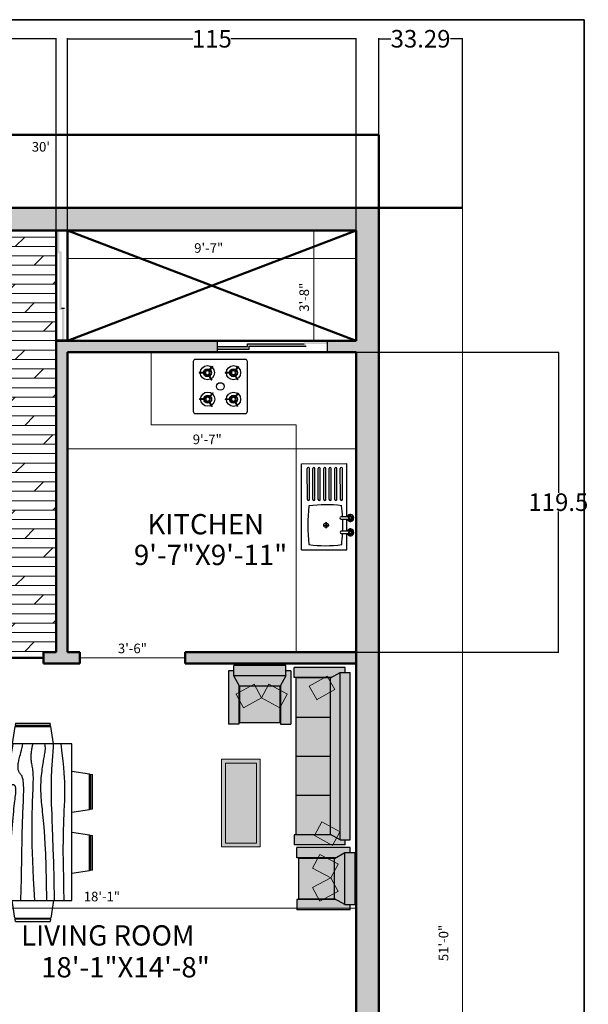
# Model space of a CAD drawing. Units: inches. Extents: x 1381 to 2246, y 1317 to 2168.
# Tile 15 of 15: x 2019 to 2246, y 1776 to 2168. Entities that reach past the tile are written whole.
import ezdxf

# ---------------------------------------------------------------- set-up
doc = ezdxf.new("R2010")
doc.units = ezdxf.units.IN
doc.header["$MEASUREMENT"] = 0
doc.layers.get('0').update_dxf_attribs({"color": 253})
for name, color, linetype, lineweight in [('A-ANNO-DIMS', 2, 'Continuous', 18), ('A-ANNO-TEXT', 7, 'Continuous', 18), ('A-ANNO-TTLB', 7, 'Continuous', 35), ('A-AREA-IDEN', 3, 'Continuous', 25), ('A-FLOR-FIXT', 9, 'Continuous', 18), ('A-FLOR-PATT', 252, 'Continuous', 13), ('A-FURN', 8, 'Continuous', 18), ('A-GLAZ', 4, 'Continuous', 25), ('A-WALL', 7, 'Continuous', 50), ('A-WALL-PATT', 8, 'Continuous', 13)]:
    doc.layers.add(name, color=color, linetype=linetype, lineweight=lineweight)
doc.layers.add('furniture', color=250, linetype='Continuous')
doc.styles.get("Standard").update_dxf_attribs({"font": 'arial.ttf'})
doc.dimstyles.get("Standard").update_dxf_attribs({"dimtxt": 7, "dimasz": 0.18, "dimexe": 0.18, "dimexo": 0.0625, "dimgap": 0.09, "dimtad": 0, "dimtih": 1, "dimtoh": 1, "dimdec": 1, "dimzin": 0, "dimdsep": 46, "dimlunit": 3, "dimtxsty": 'Standard', "dimcen": 0.09, "dimadec": 0, "dimazin": 0, "dimtfac": 1, "dimtdec": 1, "dimtofl": 0, "dimtmove": 0, "dimatfit": 3, "dimfxl": 1, "dimtolj": 1, "dimtzin": 0, "dimarcsym": 0})

# ---------------------------------------------------------------- blocks, each defined once
blk = doc.blocks.new('4bstove')
at = {"layer": 'furniture'}
for p, q in [((1452.73, 1446.21), (1452.73, 1448.61)), ((1452.98, 1446.22), (1452.98, 1448.61)), ((1464.44, 1446.34), (1464.44, 1448.73)), ((1464.69, 1446.34), (1464.69, 1448.73)), ((1451.74, 1444.45), (1449.67, 1443.25)), ((1451.87, 1444.23), (1449.79, 1443.04)), ((1453.75, 1444.08), (1455.58, 1442.54)), ((1453.91, 1444.27), (1455.74, 1442.73)), ((1463.45, 1444.58), (1461.38, 1443.38)), ((1463.57, 1444.36), (1461.5, 1443.17)), ((1465.46, 1444.21), (1467.29, 1442.67)), ((1465.62, 1444.4), (1467.45, 1442.86)), ((1452.69, 1434.81), (1452.69, 1437.2)), ((1452.94, 1434.81), (1452.94, 1437.2)), ((1464.44, 1434.81), (1464.44, 1437.2)), ((1464.69, 1434.81), (1464.69, 1437.2)), ((1451.7, 1433.04), (1449.63, 1431.85)), ((1451.82, 1432.83), (1449.75, 1431.63)), ((1453.71, 1432.67), (1455.54, 1431.13)), ((1453.87, 1432.86), (1455.7, 1431.33)), ((1463.45, 1433.04), (1461.38, 1431.85)), ((1463.57, 1432.83), (1461.5, 1431.63)), ((1465.46, 1432.67), (1467.29, 1431.13)), ((1465.62, 1432.86), (1467.45, 1431.33))]:
    blk.add_line(p, q, dxfattribs=at)
for points in [[(1447.5, 1427.38), (1469.5, 1427.38, 0.414214), (1470.5, 1428.38), (1470.5, 1450.38, 0.414214), (1469.5, 1451.38), (1447.5, 1451.38, 0.414214), (1446.5, 1450.38), (1446.5, 1428.38, 0.414214)], [(1453.75, 1444.97, 1), (1452, 1444.97, 1)], [(1465.46, 1445.1, 1), (1463.71, 1445.1, 1)], [(1453.71, 1433.56, 1), (1451.96, 1433.56, 1)], [(1465.46, 1433.56, 1), (1463.71, 1433.56, 1)]]:
    blk.add_lwpolyline(points, format="xyb", close=True, dxfattribs=at)
for points in [[(1454.12, 1444.97, 1), (1451.62, 1444.97, 1), (1454.12, 1444.97, 1)], [(1465.83, 1445.1, 1), (1463.33, 1445.1, 1), (1465.83, 1445.1, 1)], [(1454.08, 1433.56, 1), (1451.58, 1433.56, 1), (1454.08, 1433.56, 1)], [(1465.83, 1433.56, 1), (1463.33, 1433.56, 1), (1465.83, 1433.56, 1)]]:
    blk.add_lwpolyline(points, format="xyb", dxfattribs=at)
for centre, radius in [((1452.87, 1444.97), 3.14), ((1452.87, 1444.97), 1.75), ((1464.58, 1445.1), 3.14), ((1464.58, 1445.1), 1.75), ((1458.5, 1439.38), 1.67), ((1452.83, 1433.56), 3.14), ((1452.83, 1433.56), 1.75), ((1464.58, 1433.56), 3.14), ((1464.58, 1433.56), 1.75)]:
    blk.add_circle(centre, radius, dxfattribs=at)
for centre, start, end in [((1452.87, 1444.97), 88.2645, 92.2039), ((1464.58, 1445.1), 88.2645, 92.2039), ((1452.87, 1444.97), 208.188, 212.1274), ((1452.87, 1444.97), 318.1018, 322.0412), ((1464.58, 1445.1), 208.188, 212.1274), ((1464.58, 1445.1), 318.1018, 322.0412), ((1452.83, 1433.56), 88.2645, 92.2039), ((1464.58, 1433.56), 88.2645, 92.2039)]:
    blk.add_arc(centre, 3.64, start, end, dxfattribs=at)
blk = doc.blocks.new('stove')
at = {"layer": 'furniture', "xscale": 0.9, "yscale": 0.9, "zscale": 0.9, "rotation": 89.99999999999999}
blk.add_blockref('4bstove', (1295.44, -1312.65), dxfattribs=at)
blk = doc.blocks.new('A$C799204C7')
for p, q in [((0, 34.2), (17.99, 34.2)), ((0, 0), (0, 34.2)), ((2.32, 20.01), (2.32, 32.27)), ((3.13, 20.01), (3.13, 32.27)), ((4.48, 20.01), (4.48, 32.27)), ((5.29, 20.01), (5.29, 32.27)), ((6.64, 20.01), (6.64, 32.27)), ((7.45, 20.01), (7.45, 32.27)), ((8.85, 20.01), (8.85, 32.27)), ((9.66, 20.01), (9.66, 32.27)), ((11.01, 20.01), (11.01, 32.27)), ((11.82, 20.01), (11.82, 32.27)), ((13.22, 20.01), (13.22, 32.27)), ((14.03, 20.01), (14.03, 32.27)), ((15.42, 20.01), (15.42, 32.27)), ((16.24, 20.01), (16.24, 32.27)), ((17.99, 13.08), (17.99, 34.2)), ((18.59, 13.08), (15.71, 13.08)), ((15.71, 12.17), (18.59, 12.17)), ((17.99, 7.36), (17.99, 12.17)), ((8.52, 9.77), (10.9, 9.77)), ((9.73, 11), (9.73, 8.54)), ((18.59, 7.36), (15.71, 7.36)), ((15.71, 6.45), (18.59, 6.45)), ((17.99, 0), (17.99, 6.45)), ((0, 0), (17.99, 0))]:
    blk.add_line(p, q)
for centre, radius in [((19.38, 12.62), 0.684), ((19.38, 12.62), 0.456), ((9.7, 9.77), 0.916), ((19.38, 6.91), 0.684), ((19.38, 6.91), 0.456)]:
    blk.add_circle(centre, radius)
for centre, radius, start, end in [((2.72, 32.27), 0.407, 0, 180), ((4.88, 32.27), 0.407, 0, 180), ((7.05, 32.27), 0.407, 0, 180), ((9.25, 32.27), 0.407, 0, 180), ((11.42, 32.27), 0.407, 0, 180), ((13.62, 32.27), 0.407, 0, 180), ((15.83, 32.27), 0.407, 0, 180), ((2.72, 20.01), 0.407, 180, 0), ((4.88, 20.01), 0.407, 180, 0), ((7.05, 20.01), 0.407, 180, 0), ((9.25, 20.01), 0.407, 180, 0), ((11.42, 20.01), 0.407, 180, 0), ((13.62, 20.01), 0.407, 180, 0), ((15.83, 20.01), 0.407, 180, 0), ((67.33, 9.77), 64.88, 173.1952, 186.8048), ((9.53, -30.19), 48.1, 82.3437, 97.8966), ((-48.51, 9.77), 64.88, 2.9208, 6.8048), ((15.71, 12.62), 0.456, 90, 270), ((-48.51, 9.77), 64.88, 357.8723, 2.115), ((19.38, 12.62), 1.37, 199.6514, 160.3603), ((19.38, 12.62), 0.911, 210.3431, 149.7554), ((19.38, 6.91), 1.37, 199.6514, 160.3603), ((19.38, 6.91), 0.911, 210.3431, 149.7554), ((15.71, 6.91), 0.456, 90, 270), ((-48.51, 9.77), 64.88, 353.1952, 357.0665), ((9.53, 49.73), 48.1, 262.1034, 277.6563)]:
    blk.add_arc(centre, radius, start, end)
blk = doc.blocks.new('sink')
at = {"layer": 'furniture'}
for p, q in [((8718164202.684322, -1433730581.131674), (8718164202.684322, -1433730583.598095)), ((8718164203.894819, -1433730582.369047), (8718164201.504578, -1433730582.369047)), ((8718164196.150837, -1433730592.638258), (8718164196.150837, -1433730604.938997)), ((8718164196.967728, -1433730592.638258), (8718164196.967728, -1433730604.938997)), ((8718164198.365185, -1433730592.638258), (8718164198.365185, -1433730604.938997)), ((8718164199.182076, -1433730592.638258), (8718164199.182076, -1433730604.938997)), ((8718164200.579533, -1433730592.638258), (8718164200.579533, -1433730604.938997)), ((8718164201.396423, -1433730592.638258), (8718164201.396423, -1433730604.938997)), ((8718164202.748692, -1433730592.638258), (8718164202.748692, -1433730604.938997)), ((8718164203.565582, -1433730592.638258), (8718164203.565582, -1433730604.938997)), ((8718164204.963041, -1433730592.638258), (8718164204.963041, -1433730604.938997)), ((8718164205.779934, -1433730592.638258), (8718164205.779934, -1433730604.938997)), ((8718164207.1322, -1433730592.638258), (8718164207.1322, -1433730604.938997)), ((8718164207.949093, -1433730592.638258), (8718164207.949093, -1433730604.938997)), ((8718164209.301359, -1433730592.638258), (8718164209.301359, -1433730604.938997)), ((8718164210.118252, -1433730592.638258), (8718164210.118252, -1433730604.938997))]:
    blk.add_line(p, q, dxfattribs=at)
for centre, radius in [((8718164192.998869, -1433730579.495552), 0.685789), ((8718164192.998869, -1433730579.495552), 0.457192), ((8718164202.715019, -1433730582.369047), 0.919003), ((8718164192.998869, -1433730585.228166), 0.68579), ((8718164192.998869, -1433730585.228166), 0.68579), ((8718164192.998869, -1433730585.228166), 0.457192)]:
    blk.add_circle(centre, radius, dxfattribs=at)
for centre, radius, start, end in [((8718164196.559284, -1433730592.638258), 0.41045, 354.3355999, 185.6644001), ((8718164198.77363, -1433730592.638258), 0.41045, 354.3355999, 185.6644001), ((8718164200.98798, -1433730592.638258), 0.41045, 354.3355999, 185.6644001), ((8718164203.157139, -1433730592.638258), 0.41045, 354.3355999, 185.6644001), ((8718164205.371487, -1433730592.638258), 0.41045, 354.3355999, 185.6644001), ((8718164207.540646, -1433730592.640262), 0.41045, 354.3355999, 185.6644001), ((8718164209.709805, -1433730592.640262), 0.41045, 354.3355999, 185.6644001), ((8718164196.559284, -1433730604.938997), 0.408445, 180, 0), ((8718164198.77363, -1433730604.938997), 0.408445, 180, 0), ((8718164200.98798, -1433730604.938997), 0.408445, 180, 0), ((8718164203.157139, -1433730604.938997), 0.408445, 180, 0), ((8718164205.371487, -1433730604.938997), 0.408445, 180, 0), ((8718164207.540646, -1433730604.938997), 0.408445, 180, 0), ((8718164209.709805, -1433730604.938997), 0.408445, 180, 0)]:
    blk.add_arc(centre, radius, start, end, dxfattribs=at)
at = {"layer": 'furniture', "xscale": 1.0032, "yscale": 1.0032, "zscale": 1.0032, "rotation": 180}
blk.add_blockref('A$C799204C7', (8718164212.441259, -1433730572.566334), dxfattribs=at)
blk = doc.blocks.new('washbasin')
at = {"layer": 'furniture'}
blk.add_blockref('sink', (-8718164214.119328, 1433730589.721069), dxfattribs=at)
blk = doc.blocks.new('Dining Set - 36 x 72 in.')
for p, q in [((-22, 27.5), (-22.1562, 26.50042)), ((-22, 27.5), (-6, 27.5)), ((-5.8437, 26.49966), (-6, 27.5)), ((6, 27.5), (5.8438, 26.50042)), ((6, 27.5), (22, 27.5)), ((22.1563, 26.49966), (22, 27.5)), ((-22.2343, 26.00059), (-23.4847, 17.99762)), ((-22.2304, 26), (-5.7608, 26)), ((-5.8416, 26.5), (-22.1534, 26.5)), ((-4.5152, 17.99762), (-5.7655, 25.99926)), ((5.7657, 26.00059), (4.5153, 17.99762)), ((5.7696, 26), (22.2392, 26)), ((22.1584, 26.5), (5.8466, 26.5)), ((23.4848, 17.99762), (22.2345, 25.99926)), ((36, 18), (-36, 18)), ((-36, 18), (-36, -18)), ((36, -18), (36, 18)), ((-44.0006, 8.23428), (-35.9976, 9.48474)), ((44.0006, 8.23428), (35.9976, 9.48474)), ((-45.5, 8), (-44.5004, 8.15617)), ((-45.5, 8), (-45.5, -8)), ((-44.5, -8.15843), (-44.5, 8.15338)), ((-44, 8.23041), (-44, -8.23915)), ((44, 8.23041), (44, -8.23915)), ((44.5, -8.15843), (44.5, 8.15338)), ((45.5, 8), (44.5005, 8.15617)), ((45.5, 8), (45.5, -8)), ((-44.4997, -8.15631), (-45.5, -8)), ((-35.9976, -9.48476), (-43.9993, -8.2345)), ((35.9976, -9.48476), (43.9993, -8.2345)), ((44.4997, -8.15631), (45.5, -8)), ((-36, -18), (36, -18)), ((-22.2343, -26.0006), (-23.4847, -17.99762)), ((-4.5152, -17.99762), (-5.7655, -25.99928)), ((5.7657, -26.0006), (4.5153, -17.99762)), ((23.4848, -17.99762), (22.2345, -25.99928)), ((-22.2304, -26), (-5.7608, -26)), ((-22, -27.5), (-22.1562, -26.50044)), ((-5.8416, -26.5), (-22.1534, -26.5)), ((-5.8437, -26.49967), (-6, -27.5)), ((5.7696, -26), (22.2392, -26)), ((6, -27.5), (5.8438, -26.50044)), ((22.1584, -26.5), (5.8466, -26.5)), ((22.1563, -26.49967), (22, -27.5)), ((-22, -27.5), (-6, -27.5)), ((6, -27.5), (22, -27.5))]:
    blk.add_line(p, q)
for points in [[(-36, 15), (-31.1772, 14.97754), (-26.8079, 14.91406), (-22.8538, 14.81543), (-19.276, 14.6875), (-16.0362, 14.53613), (-13.0957, 14.36718), (-10.4159, 14.18652), (-7.9583, 14), (-5.6904, 13.81315), (-3.6035, 13.63021), (-1.6954, 13.45508), (0.0365, 13.29166), (1.5945, 13.14388), (2.9811, 13.01562), (4.1988, 12.9108), (5.25, 12.83333), (6.1393, 12.78613), (6.8802, 12.76823), (7.4883, 12.77767), (7.9792, 12.8125), (8.3685, 12.87077), (8.6719, 12.95052), (8.9049, 13.0498), (9.0833, 13.16666), (9.2205, 13.29899), (9.3216, 13.44401), (9.3895, 13.59879), (9.4271, 13.76041), (9.4373, 13.92594), (9.4232, 14.09245), (9.3875, 14.257), (9.3333, 14.41666), (9.2638, 14.56917), (9.1836, 14.71484), (9.0975, 14.85465), (9.0104, 14.98958), (8.9272, 15.1206), (8.8529, 15.2487), (8.7922, 15.37483), (8.75, 15.5), (8.7305, 15.62467), (8.7344, 15.74739), (8.7617, 15.86621), (8.8125, 15.97916), (8.8867, 16.08431), (8.9844, 16.17968), (9.1055, 16.26334), (9.25, 16.33333), (9.4189, 16.38802), (9.6172, 16.42708), (9.8506, 16.45052), (10.125, 16.45833), (10.4463, 16.45052), (10.8203, 16.42708), (11.2529, 16.38802), (11.75, 16.33333), (12.3184, 16.26318), (12.9694, 16.17838), (13.7151, 16.07991), (14.5677, 15.96875), (15.5395, 15.84586), (16.6426, 15.71224), (17.8893, 15.56884), (19.2917, 15.41666), (20.859, 15.25667), (22.5879, 15.08984), (24.4721, 14.91715), (26.5052, 14.73958), (28.6809, 14.5581), (30.9929, 14.3737), (33.4347, 14.18733), (36, 14)], [(-36, 10), (-28.9766, 10.14274), (-23.1725, 10.20442), (-18.4241, 10.19775), (-14.5677, 10.13541), (-11.4399, 10.03011), (-8.877, 9.89453), (-6.7154, 9.74137), (-4.7917, 9.58333), (-2.9698, 9.43082), (-1.2246, 9.28515), (0.4415, 9.14534), (2.026, 9.01041), (3.5266, 8.87939), (4.9408, 8.7513), (6.266, 8.62516), (7.5, 8.5), (8.6411, 8.37549), (9.6914, 8.2539), (10.6538, 8.13818), (11.5312, 8.03125), (12.3267, 7.93603), (13.043, 7.85547), (13.6831, 7.79248), (14.25, 7.75), (14.7471, 7.7303), (15.1797, 7.73307), (15.5537, 7.75732), (15.875, 7.80208), (16.1494, 7.86637), (16.3828, 7.94922), (16.5811, 8.04964), (16.75, 8.16666), (16.8944, 8.29915), (17.0143, 8.44531), (17.1089, 8.60319), (17.1771, 8.77083), (17.218, 8.94629), (17.2305, 9.1276), (17.2137, 9.31282), (17.1667, 9.5), (17.0895, 9.6875), (16.987, 9.875), (16.8649, 10.0625), (16.7292, 10.25), (16.5856, 10.4375), (16.4401, 10.625), (16.2985, 10.8125), (16.1667, 11), (16.05, 11.18733), (15.9518, 11.3737), (15.8752, 11.5581), (15.8229, 11.73958), (15.798, 11.91715), (15.8034, 12.08984), (15.842, 12.25667), (15.9167, 12.41666), (16.0295, 12.56836), (16.1784, 12.70833), (16.3605, 12.83268), (16.5729, 12.9375), (16.8127, 13.01888), (17.0768, 13.07291), (17.3625, 13.0957), (17.6667, 13.08333), (17.9894, 13.03312), (18.3418, 12.94726), (18.7382, 12.82918), (19.1927, 12.68229), (19.7195, 12.51001), (20.3327, 12.31575), (21.0465, 12.10294), (21.875, 11.875), (22.8357, 11.63354), (23.959, 11.37304), (25.2786, 11.08618), (26.8282, 10.76562), (28.6414, 10.40405), (30.752, 9.99414), (33.1936, 9.52856), (36, 9)], [(-36, 5.5), (-30.7157, 5.3348), (-26.069, 5.20963), (-21.9946, 5.11767), (-18.4271, 5.05208), (-15.3009, 5.00602), (-12.5508, 4.97265), (-10.1112, 4.94515), (-7.9167, 4.91666), (-5.909, 4.88167), (-4.0586, 4.83984), (-2.3429, 4.79215), (-0.7396, 4.73958), (0.7739, 4.6831), (2.22, 4.6237), (3.6213, 4.56233), (5, 4.5), (6.373, 4.43782), (7.7344, 4.3776), (9.0723, 4.32129), (10.375, 4.27083), (11.6309, 4.22819), (12.8281, 4.19531), (13.9551, 4.17415), (15, 4.16666), (15.954, 4.17448), (16.819, 4.19791), (17.6001, 4.23698), (18.3021, 4.29166), (18.9299, 4.36198), (19.4883, 4.44791), (19.9823, 4.54948), (20.4167, 4.66666), (20.7969, 4.79899), (21.1302, 4.94401), (21.4245, 5.09879), (21.6875, 5.26041), (21.9271, 5.42594), (22.1511, 5.59245), (22.3672, 5.757), (22.5834, 5.91666), (22.8065, 6.06868), (23.0404, 6.21093), (23.2879, 6.34147), (23.5521, 6.45833), (23.8358, 6.55957), (24.142, 6.64323), (24.4735, 6.70735), (24.8334, 6.75), (25.2235, 6.76969), (25.642, 6.76692), (26.0858, 6.74267), (26.5521, 6.69791), (27.0379, 6.63362), (27.5404, 6.55078), (28.0565, 6.45036), (28.5834, 6.33333), (29.1242, 6.19987), (29.7071, 6.04687), (30.3661, 5.87044), (31.1354, 5.66666), (32.0493, 5.43164), (33.142, 5.16146), (34.4475, 4.85221), (36, 4.5)], [(-36, -1), (-30.7915, -0.6591), (-26.0195, -0.38216), (-21.6519, -0.16284), (-17.6563, 0.00521), (-14.0005, 0.12833), (-10.6523, 0.21289), (-7.5796, 0.26522), (-4.75, 0.29166), (-2.134, 0.29793), (0.2878, 0.28711), (2.5317, 0.26163), (4.6146, 0.22396), (6.5529, 0.17651), (8.3633, 0.12174), (10.0623, 0.06209), (11.6667, 0), (13.1899, -0.06201), (14.6341, -0.1211), (15.9982, -0.17432), (17.2813, -0.21875), (18.4823, -0.25147), (19.6003, -0.26953), (20.6343, -0.27002), (21.5834, -0.25), (22.4481, -0.20768), (23.2357, -0.14584), (23.9549, -0.06836), (24.6146, 0.02083), (25.2235, 0.11784), (25.7904, 0.21875), (26.3241, 0.31966), (26.8334, 0.41666), (27.3265, 0.50618), (27.8099, 0.58593), (28.2894, 0.65397), (28.7709, 0.70833), (29.2601, 0.74707), (29.763, 0.76823), (30.2855, 0.76985), (30.8334, 0.75), (31.4088, 0.70784), (31.9994, 0.64713), (32.589, 0.57275), (33.1615, 0.48958), (33.7008, 0.4025), (34.1908, 0.3164), (34.6153, 0.23616), (34.9584, 0.16666), (35.2099, 0.11165), (35.3848, 0.07031), (35.504, 0.04069), (35.5886, 0.02083), (35.6594, 0.00879), (35.7377, 0.0026), (35.8442, 0.00032), (36, 0)], [(-36, -6.5), (-27.1843, -6.31267), (-20.084, -6.1263), (-14.469, -5.9419), (-10.1094, -5.76042), (-6.7752, -5.58285), (-4.2363, -5.41016), (-2.2629, -5.24333), (-0.625, -5.08334), (0.8708, -4.93099), (2.2715, -4.78646), (3.5872, -4.64974), (4.8281, -4.52084), (6.0046, -4.39974), (7.127, -4.28646), (8.2053, -4.18099), (9.25, -4.08334), (10.2705, -3.99382), (11.2734, -3.91407), (12.2647, -3.84603), (13.25, -3.79167), (14.2354, -3.75293), (15.2266, -3.73177), (16.2295, -3.73015), (17.25, -3.75), (18.2912, -3.79248), (19.3451, -3.85547), (20.4009, -3.93604), (21.4479, -4.03125), (22.4754, -4.13819), (23.4727, -4.25391), (24.4289, -4.37549), (25.3334, -4.5), (26.1785, -4.62492), (26.9694, -4.74935), (27.7145, -4.87281), (28.4219, -4.99479), (29.1, -5.11483), (29.7572, -5.23242), (30.4016, -5.34709), (31.0417, -5.45834), (31.6837, -5.56437), (32.3262, -5.65821), (32.9658, -5.73153), (33.599, -5.77604), (34.2224, -5.78345), (34.8327, -5.74545), (35.4264, -5.65373), (36, -5.5)], [(-36, -10), (-26.4022, -9.81299), (-18.4675, -9.62891), (-11.9839, -9.45069), (-6.7396, -9.28125), (-2.5226, -9.12354), (0.8789, -8.98047), (3.6769, -8.85498), (6.0833, -8.75), (8.2767, -8.66765), (10.3021, -8.60677), (12.1712, -8.56543), (13.8958, -8.54167), (15.4876, -8.53353), (16.9583, -8.53907), (18.3197, -8.55632), (19.5834, -8.58334), (20.7616, -8.61841), (21.8685, -8.66081), (22.9188, -8.71004), (23.9271, -8.76563), (24.9081, -8.82707), (25.8763, -8.89388), (26.8465, -8.96558), (27.8334, -9.04167), (28.8474, -9.12118), (29.8828, -9.20117), (30.93, -9.27824), (31.9792, -9.34896), (33.0205, -9.40991), (34.0443, -9.45768), (35.0407, -9.48885), (36, -9.5)], [(-36, -14.5), (-30.0881, -14.33513), (-25.0332, -14.21224), (-20.7312, -14.12647), (-17.0781, -14.07292), (-13.97, -14.04671), (-11.3027, -14.04297), (-8.9724, -14.05681), (-6.875, -14.08334), (-4.9224, -14.11833), (-3.0905, -14.16016), (-1.3709, -14.20785), (0.2448, -14.26042), (1.7647, -14.3169), (3.1973, -14.3763), (4.5507, -14.43767), (5.8333, -14.5), (7.0554, -14.5621), (8.235, -14.62175), (9.3922, -14.67652), (10.5469, -14.72396), (11.7192, -14.76164), (12.929, -14.78711), (14.1965, -14.79794), (15.5417, -14.79167), (16.9933, -14.76424), (18.6152, -14.70508), (20.4804, -14.60197), (22.6615, -14.44271), (25.2312, -14.21509), (28.2624, -13.9069), (31.8277, -13.50594), (36, -13)]]:
    blk.add_lwpolyline(points)
blk = doc.blocks.new('dining area')
at = {"layer": 'furniture', "xscale": 0.6659924291999282, "yscale": 0.6659924291999282, "zscale": 0.6659924291999282, "rotation": 90}
blk.add_blockref('Dining Set - 36 x 72 in.', (-0.44, 20.51), dxfattribs=at)
blk = doc.blocks.new('FABRIC SOFA 4S')
at = {"layer": 'furniture'}
for p, q in [((3, 54), (34, 54)), ((3, 51), (3, 54)), ((34, 48), (34, 54)), ((0, -51), (0, 51)), ((6, 51), (0, 51)), ((6, -51), (6, 51)), ((12, 47.63), (6, 51)), ((11.14, 48), (34, 48)), ((33, 23.81), (12, 23.81)), ((33, 0), (12, 0)), ((33, -23.81), (12, -23.81)), ((6, -51), (12, -47.63)), ((6, -51), (0, -51)), ((3, -54), (3, -51)), ((11.54, -48), (34, -48)), ((34, -48), (34, -54)), ((3, -54), (34, -54))]:
    blk.add_line(p, q, dxfattribs=at)
blk.add_lwpolyline([(12, -47.63), (12, 47.63), (33, 47.63), (33, -47.63)], close=True, dxfattribs=at)
blk = doc.blocks.new('FABRIC SOFA 1S')
at = {"layer": 'furniture'}
for p, q in [((3, 18.12), (34, 18.12)), ((3, 15.12), (3, 18.12)), ((34, 12.12), (34, 18.12)), ((0, -15.12), (0, 15.12)), ((6, 15.12), (0, 15.12)), ((6, -15.12), (6, 15.12)), ((12, 11.75), (6, 15.12)), ((11.33, 12.12), (34, 12.12)), ((6, -15.12), (0, -15.12)), ((3, -18.12), (3, -15.12)), ((6, -15.12), (12, -11.75)), ((11.33, -12.12), (34, -12.12)), ((34, -12.12), (34, -18.12)), ((3, -18.12), (34, -18.12))]:
    blk.add_line(p, q, dxfattribs=at)
blk.add_lwpolyline([(12, -11.75), (12, 11.75), (33, 11.75), (33, -11.75)], close=True, dxfattribs=at)
blk = doc.blocks.new('TV-UNIT')
for p, q in [((0, 5.36), (7.38, 9.32)), ((7.38, 9.32), (10.3, 3.88)), ((13.22, 9.32), (10.3, 3.88)), ((20.6, 5.36), (13.22, 9.32)), ((3.07, 0), (0.15, 5.44)), ((17.53, 0), (20.45, 5.44)), ((10.3, 3.88), (3.07, 0)), ((10.3, 3.88), (17.53, 0))]:
    blk.add_line(p, q)
blk = doc.blocks.new('WALL-UNIT')
for p, q in [((2.92, 18.64), (0, 13.2)), ((10.3, 14.68), (2.92, 18.64)), ((0, 13.2), (7.23, 9.32)), ((7.23, 9.32), (10.15, 14.76)), ((0, 5.44), (7.23, 9.32)), ((7.23, 9.32), (10.15, 3.88)), ((2.92, 0), (0, 5.44)), ((10.3, 3.96), (2.92, 0))]:
    blk.add_line(p, q)
blk = doc.blocks.new('SOFA-CUSHION')
for p, q in [((2.92, 9.32), (0, 3.88)), ((10.3, 5.36), (2.92, 9.32)), ((7.23, 0), (10.15, 5.44)), ((0, 3.88), (7.23, 0))]:
    blk.add_line(p, q)
blk = doc.blocks.new('WIN-KITCHEN')
for p, q in [((0, 0), (0, 4.5)), ((0, 4.5), (43.68, 4.5)), ((43.68, 4.5), (43.68, 0)), ((43.68, 0), (0, 0))]:
    blk.add_line(p, q)
blk = doc.blocks.new('CENTER-TABLE')
for p, q in [((0, 0), (0, 34.91)), ((0, 34.91), (15.37, 34.91)), ((15.37, 34.91), (15.37, 0)), ((15.37, 0), (0, 0))]:
    blk.add_line(p, q)
blk = doc.blocks.new('SIDE-TABLE')
for p, q in [((0, 0), (0, 31.87)), ((0, 31.87), (12.34, 31.87)), ((12.34, 31.87), (12.34, 0)), ((12.34, 0), (0, 0))]:
    blk.add_line(p, q)
blk = doc.blocks.new('*D78')
at = {"layer": 'A-ANNO-DIMS', "color": 0, "lineweight": -2, "transparency": 16777216}
for p, q in [((2162.31, 2092.98), (2162.31, 2160.41)), ((2162.49, 2160.23), (2167.04, 2160.23)), ((2195.41, 2160.23), (2190.86, 2160.23)), ((2195.59, 2092.98), (2195.59, 2160.41))]:
    blk.add_line(p, q, dxfattribs=at)
at = {"layer": 'A-ANNO-DIMS', "color": 0, "transparency": 16777216}
for points in [[(2162.49, 2160.26), (2162.49, 2160.2), (2162.31, 2160.23)], [(2195.41, 2160.26), (2195.41, 2160.2), (2195.59, 2160.23)]]:
    blk.add_solid(points, dxfattribs=at)
at = {"layer": 'Defpoints', "color": 0, "transparency": 16777216}
for p in [(2195.59, 2160.23), (2162.31, 2092.92), (2195.59, 2092.92)]:
    blk.add_point(p, dxfattribs=at)
at = {"layer": 'A-ANNO-DIMS', "color": 0, "transparency": 16777216, "insert": (2178.95, 2160.23), "char_height": 7, "attachment_point": 5}
blk.add_mtext('\\A1;33.29', dxfattribs=at)
blk = doc.blocks.new('*D84')
at = {"layer": 'A-ANNO-DIMS', "color": 0, "lineweight": -2, "transparency": 16777216}
for p, q in [((1871.81, 2083.98), (1871.81, 2160.41)), ((1871.99, 2160.23), (1945.35, 2160.23)), ((2033.63, 2160.23), (1960.26, 2160.23)), ((2033.81, 2083.98), (2033.81, 2160.41))]:
    blk.add_line(p, q, dxfattribs=at)
at = {"layer": 'A-ANNO-DIMS', "color": 0, "transparency": 16777216}
for points in [[(1871.99, 2160.26), (1871.99, 2160.2), (1871.81, 2160.23)], [(2033.63, 2160.26), (2033.63, 2160.2), (2033.81, 2160.23)]]:
    blk.add_solid(points, dxfattribs=at)
at = {"layer": 'Defpoints', "color": 0, "transparency": 16777216}
for p in [(2033.81, 2160.23), (1871.81, 2083.92), (2033.81, 2083.92)]:
    blk.add_point(p, dxfattribs=at)
at = {"layer": 'A-ANNO-DIMS', "color": 0, "transparency": 16777216, "insert": (1952.81, 2160.23), "char_height": 7, "attachment_point": 5}
blk.add_mtext('\\A1;162', dxfattribs=at)
blk = doc.blocks.new('*D85')
at = {"layer": 'A-ANNO-DIMS', "color": 0, "lineweight": -2, "transparency": 16777216}
for p, q in [((2038.31, 2083.98), (2038.31, 2160.41)), ((2038.49, 2160.23), (2088.29, 2160.23)), ((2153.13, 2160.23), (2103.32, 2160.23)), ((2153.31, 2083.98), (2153.31, 2160.41))]:
    blk.add_line(p, q, dxfattribs=at)
at = {"layer": 'A-ANNO-DIMS', "color": 0, "transparency": 16777216}
for points in [[(2038.49, 2160.26), (2038.49, 2160.2), (2038.31, 2160.23)], [(2153.13, 2160.26), (2153.13, 2160.2), (2153.31, 2160.23)]]:
    blk.add_solid(points, dxfattribs=at)
at = {"layer": 'Defpoints', "color": 0, "transparency": 16777216}
for p in [(2153.31, 2160.23), (2038.31, 2083.92), (2153.31, 2083.92)]:
    blk.add_point(p, dxfattribs=at)
at = {"layer": 'A-ANNO-DIMS', "color": 0, "transparency": 16777216, "insert": (2095.81, 2160.23), "char_height": 7, "attachment_point": 5}
blk.add_mtext('\\A1;115', dxfattribs=at)
blk = doc.blocks.new('*D87')
at = {"layer": 'A-ANNO-DIMS', "color": 0, "lineweight": -2, "transparency": 16777216}
for p, q in [((2153.37, 2035.42), (2234.02, 2035.42)), ((2233.84, 2035.24), (2233.84, 1979.33)), ((2233.84, 1916.1), (2233.84, 1972)), ((2153.37, 1915.92), (2234.02, 1915.92))]:
    blk.add_line(p, q, dxfattribs=at)
at = {"layer": 'A-ANNO-DIMS', "color": 0, "transparency": 16777216}
for points in [[(2233.81, 2035.24), (2233.87, 2035.24), (2233.84, 2035.42)], [(2233.81, 1916.1), (2233.87, 1916.1), (2233.84, 1915.92)]]:
    blk.add_solid(points, dxfattribs=at)
at = {"layer": 'Defpoints', "color": 0, "transparency": 16777216}
for p in [(2153.31, 2035.42), (2233.84, 2035.42), (2153.31, 1915.92)]:
    blk.add_point(p, dxfattribs=at)
at = {"layer": 'A-ANNO-DIMS', "color": 0, "transparency": 16777216, "insert": (2233.84, 1975.67), "char_height": 7, "attachment_point": 5}
blk.add_mtext('\\A1;119.5', dxfattribs=at)

msp = doc.modelspace()

# ---------------------------------------------------------------- hatches: boundary and pattern name
at = {"layer": 'A-FLOR-PATT'}
h = msp.add_hatch(dxfattribs=at)
h.set_pattern_fill('DOLMIT', color=256, scale=15)
h.paths.add_polyline_path([(2033.8052, 2083.9163), (1932.8359, 2083.9163), (1932.8359, 2057.4148), (1871.8052, 2057.4148), (1871.8052, 1915.9163), (1900.7902, 1915.9163), (1900.7902, 1913.6663), (1929.807, 1913.6663), (1929.807, 1915.9163), (1990.4785, 1915.9163), (1990.4785, 1913.6663), (2028.7731, 1913.6663), (2028.7731, 1915.9163), (2033.8052, 1915.9163)])
edge = h.paths.add_edge_path(flags=16)
edge.add_spline(control_points=[(1939.5401, 1955.9789), (1939.5923, 1955.9054), (1939.7074, 1955.7434), (1939.52, 1955.4418), (1939.2609, 1955.0703), (1939.5201, 1954.8623), (1939.6513, 1954.757)], knot_values=[0, 0, 0, 0, 0.37399428, 0.82431366, 1.46117297, 2.11445126, 2.11445126, 2.11445126, 2.11445126], degree=3, periodic=0)
edge.add_spline(control_points=[(1939.8748, 1955.9789), (1939.9271, 1955.9054), (1940.0422, 1955.7434), (1939.8548, 1955.4418), (1939.5956, 1955.0703), (1939.8548, 1954.8623), (1939.986, 1954.757)], knot_values=[0, 0, 0, 0, 0.37399428, 0.82431366, 1.46117297, 2.11445126, 2.11445126, 2.11445126, 2.11445126], degree=3, periodic=0)
edge = h.paths.add_edge_path(flags=16)
edge.add_line((1942.0171, 2024.4608), (1942.0171, 1955.9789))
edge.add_line((1942.0171, 1955.9789), (1913.4617, 1955.9789))
edge.add_line((1913.4617, 1955.9789), (1913.4617, 1962.7697))
edge.add_line((1913.4617, 1962.7697), (1887.334, 1962.7697))
edge.add_line((1887.334, 1962.7697), (1887.445, 1951.263))
edge.add_line((1887.445, 1951.263), (1874.2492, 1951.263))
edge.add_line((1874.2492, 1951.263), (1874.1382, 1962.7697))
edge.add_line((1874.1382, 1962.7697), (1874.1382, 2014.1291))
edge.add_line((1874.1382, 2014.1291), (1874.0273, 2025.6358))
edge.add_line((1874.0273, 2025.6358), (1887.2231, 2025.6358))
edge.add_line((1887.2231, 2025.6358), (1887.334, 2014.1291))
edge.add_line((1887.334, 2014.1291), (1913.4617, 2014.1291))
edge.add_line((1913.4617, 2014.1291), (1913.4617, 2024.4608))
edge.add_line((1913.4617, 2024.4608), (1939.579, 2024.4608))
edge.add_spline(control_points=[(1939.579, 2024.4608), (1939.6269, 2024.5305), (1939.736, 2024.6891), (1939.5499, 2024.9858), (1939.2914, 2025.3575), (1939.5505, 2025.5655), (1939.6817, 2025.6708)], knot_values=[0, 0, 0, 0, 0.3521435, 0.80246288, 1.43932219, 2.09260048, 2.09260048, 2.09260048, 2.09260048], degree=3, periodic=0)
edge.add_spline(control_points=[(1940.0164, 2025.6708), (1939.8852, 2025.5655), (1939.6261, 2025.3575), (1939.8847, 2024.9858), (1940.0707, 2024.6891), (1939.9616, 2024.5305), (1939.9137, 2024.4608)], knot_values=[0, 0, 0, 0, 0.65327829, 1.2901376, 1.74045698, 2.09260048, 2.09260048, 2.09260048, 2.09260048], degree=3, periodic=0)
edge.add_line((1939.9137, 2024.4608), (1942.0171, 2024.4608))
h.paths.add_polyline_path([(1891.698, 2014.0737), (1891.698, 2004.8072), (1884.8656, 2004.8072), (1884.8197, 2004.7449), (1884.8197, 1968.5691), (1877.0588, 1968.5691), (1877.0588, 1983.6181), (1884.8197, 1983.6181), (1884.8197, 1989.7582), (1877.0588, 1989.7582), (1877.0588, 2004.8072), (1884.8656, 2004.8072)], flags=0)
h.paths.add_polyline_path([(1884.8729, 2020.1923, -1), (1876.3774, 2020.1923, -1)], flags=0)
h.paths.add_polyline_path([(1884.9838, 1957.3262, -1), (1876.4884, 1957.3262, -1)], flags=0)
h.paths.add_polyline_path([(1949.3287, 1985.8776), (2018.4467, 1985.8776), (2018.4467, 1998.2538), (1949.3287, 1998.2538)], flags=24)
h.paths.add_polyline_path([(1951.1032, 2002.3157), (2019.8384, 2002.3157), (2019.8384, 2014.8488), (1951.1032, 2014.8488)], flags=24)
at = {"layer": 'A-FURN'}
h = msp.add_hatch(color=256, dxfattribs=at)
h.dxf.hatch_style = 1
h.paths.add_polyline_path([(2122.9656, 1902.3282), (2106.8553, 1902.3282), (2106.8553, 1887.9317), (2122.9656, 1887.9317)])
h.paths.add_polyline_path([(2125.2793, 1906.4414), (2104.5416, 1906.4414), (2106.8553, 1902.3282), (2122.9656, 1902.3282)])
h.paths.add_polyline_path([(2125.2793, 1910.5547), (2104.5416, 1910.5547), (2104.5416, 1906.4414), (2125.2793, 1906.4414)])
h.paths.add_polyline_path([(2106.5982, 1902.7852), (2104.5416, 1906.4414), (2104.5416, 1908.4981), (2102.485, 1908.4981), (2102.485, 1887.2462), (2106.5982, 1887.2462)])
h.paths.add_polyline_path([(2127.336, 1908.4981), (2125.2793, 1908.4981), (2125.2793, 1906.4414), (2123.2227, 1902.7852), (2123.2227, 1887.2462), (2127.336, 1887.2462)])
h = msp.add_hatch(color=256, dxfattribs=at)
h.dxf.hatch_style = 1
h.paths.add_polyline_path([(2146.9652, 1907.8492), (2148.9266, 1907.8492), (2148.9266, 1909.8106), (2128.659, 1909.8106), (2128.659, 1905.8878), (2143.4783, 1905.8878)])
h.paths.add_polyline_path([(2143.0425, 1905.6427), (2129.3128, 1905.6427), (2129.3128, 1890.0742), (2143.0425, 1890.0742)])
h.paths.add_polyline_path([(2143.0425, 1890.0742), (2129.3128, 1890.0742), (2129.3128, 1874.5057), (2143.0425, 1874.5057)])
h.paths.add_polyline_path([(2143.0425, 1874.5057), (2129.3128, 1874.5057), (2129.3128, 1858.9372), (2143.0425, 1858.9372)])
h = msp.add_hatch(color=256, dxfattribs=at)
h.dxf.hatch_style = 1
h.paths.add_polyline_path([(2150.888, 1907.8492), (2146.9652, 1907.8492), (2146.9652, 1841.1622), (2150.888, 1841.1622)])
h.paths.add_polyline_path([(2146.9652, 1907.8492), (2143.0425, 1905.6427), (2143.0425, 1843.3688), (2146.9652, 1841.1622)])
h.paths.add_polyline_path([(2143.0425, 1858.9372), (2129.3128, 1858.9372), (2129.3128, 1843.3688), (2143.0425, 1843.3688)])
h.paths.add_polyline_path([(2146.9652, 1841.1622), (2143.4783, 1843.1236), (2128.659, 1843.1236), (2128.659, 1839.2008), (2148.9266, 1839.2008), (2148.9266, 1841.1622)])
h = msp.add_hatch(color=256, dxfattribs=at)
h.dxf.hatch_style = 1
h.paths.add_polyline_path([(2137.3321, 1897.028), (2144.5643, 1900.9083), (2141.6465, 1906.3465), (2134.4144, 1902.4662)])
h = msp.add_hatch(color=256, dxfattribs=at)
h.dxf.hatch_style = 1
h.paths.add_polyline_path([(2112.6926, 1903.1174), (2105.4604, 1899.2371), (2108.3782, 1893.799), (2115.6103, 1897.6793)])
h = msp.add_hatch(color=256, dxfattribs=at)
h.dxf.hatch_style = 1
h.paths.add_polyline_path([(2118.5281, 1903.1174), (2125.7603, 1899.2371), (2122.8425, 1893.799), (2115.6103, 1897.6793)])
h = msp.add_hatch(color=256, dxfattribs=at)
h.dxf.hatch_style = 1
h.paths.add_polyline_path([(2115.0701, 1873.2707), (2099.6959, 1873.2707), (2099.6959, 1838.3593), (2115.0701, 1838.3593)])
h.paths.add_polyline_path([(2101.2152, 1871.7514), (2113.5508, 1871.7514), (2113.5508, 1839.8786), (2101.2152, 1839.8786)], flags=16)
h = msp.add_hatch(color=256, dxfattribs=at)
h.dxf.hatch_style = 1
h.paths.add_polyline_path([(2113.5508, 1871.7514), (2101.2152, 1871.7514), (2101.2152, 1839.8786), (2113.5508, 1839.8786)])
h = msp.add_hatch(color=256, dxfattribs=at)
h.dxf.hatch_style = 1
h.paths.add_polyline_path([(2139.5829, 1848.2968), (2146.8151, 1844.4165), (2143.8973, 1838.9783), (2136.6651, 1842.8586)])
h = msp.add_hatch(color=256, dxfattribs=at)
h.dxf.hatch_style = 1
h.paths.add_polyline_path([(2150.888, 1838.1626), (2129.6361, 1838.1626), (2129.6361, 1834.0493), (2145.1751, 1834.0493), (2148.8314, 1836.106), (2150.888, 1836.106)])
h.paths.add_polyline_path([(2144.7181, 1833.7922), (2130.3217, 1833.7922), (2130.3217, 1817.6819), (2144.7181, 1817.6819)])
h.paths.add_polyline_path([(2150.888, 1815.3682), (2148.8314, 1815.3682), (2145.1751, 1817.4249), (2129.6361, 1817.4249), (2129.6361, 1813.3116), (2150.888, 1813.3116)])
h.paths.add_polyline_path([(2148.8314, 1836.106), (2144.7181, 1833.7922), (2144.7181, 1817.6819), (2148.8314, 1815.3682)])
h.paths.add_polyline_path([(2152.9446, 1836.106), (2148.8314, 1836.106), (2148.8314, 1815.3682), (2152.9446, 1815.3682)])
h = msp.add_hatch(color=256, dxfattribs=at)
h.dxf.hatch_style = 1
h.paths.add_polyline_path([(2138.8531, 1835.4011), (2146.0853, 1831.5208), (2143.1676, 1826.0827), (2135.9354, 1829.963)])
h = msp.add_hatch(color=256, dxfattribs=at)
h.dxf.hatch_style = 1
h.paths.add_polyline_path([(2138.8531, 1816.7642), (2146.0853, 1820.6445), (2143.1676, 1826.0827), (2135.9354, 1822.2024)])
at = {"layer": 'A-GLAZ'}
h = msp.add_hatch(color=256, dxfattribs=at)
h.dxf.hatch_style = 1
h.paths.add_polyline_path([(2035.919, 2052.8139), (2035.919, 2075.5544), (2035.0827, 2075.5544), (2035.0827, 2083.9163), (2034.4207, 2083.9163), (2034.4207, 2074.7522), (2035.0131, 2074.7522), (2035.0131, 2052.1861), (2036.0552, 2052.1861), (2036.0552, 2040.2358), (2037.0689, 2040.2358), (2037.0689, 2052.8139)])
h = msp.add_hatch(color=256, dxfattribs=at)
h.dxf.hatch_style = 1
h.paths.add_polyline_path([(2110.6154, 2037.8025), (2133.3559, 2037.8025), (2133.3559, 2038.6388), (2141.7178, 2038.6388), (2141.7178, 2039.3008), (2132.5537, 2039.3008), (2132.5537, 2038.7085), (2109.9876, 2038.7085), (2109.9876, 2037.6663), (2098.0373, 2037.6663), (2098.0373, 2036.6526), (2110.6154, 2036.6526)])
at = {"layer": 'A-WALL-PATT'}
h = msp.add_hatch(color=256, dxfattribs=at)
h.dxf.hatch_style = 1
h.paths.add_polyline_path([(1990.4785, 1915.9163), (1929.807, 1915.9163), (1929.807, 1911.4163), (1990.4785, 1911.4163)], flags=17)
h.paths.add_polyline_path([(1900.7902, 1915.9163), (1871.8052, 1915.9163), (1871.8052, 1911.4163), (1900.7902, 1911.4163)], flags=17)
h.paths.add_polyline_path([(2043.2216, 1915.9163), (2038.3052, 1915.9163), (2038.3052, 2035.4163), (2098.0373, 2035.4163), (2098.0373, 2039.9163), (2033.8052, 2039.9163), (2033.8052, 1915.9163), (2028.7731, 1915.9163), (2028.7731, 1911.4163), (2043.2216, 1911.4163)], flags=17)
h.paths.add_polyline_path([(2153.3052, 1915.9163), (2085.2216, 1915.9163), (2085.2216, 1911.4163), (2153.3052, 1911.4163)], flags=17)
h.paths.add_polyline_path([(1935.508, 1911.4163), (1931.008, 1911.4163), (1931.008, 1779.4163), (1899.8394, 1779.4163), (1899.8394, 1774.9163), (1902.8052, 1774.9163), (1979.3052, 1774.9163), (1979.3052, 1770.3401), (1983.8052, 1770.3401), (1983.8052, 1779.4163), (1935.508, 1779.4163)], flags=17)
h.paths.add_polyline_path([(1871.8052, 2083.9163), (2153.3052, 2083.9163), (2153.3052, 2039.9163), (2141.7178, 2039.9163), (2141.7178, 2035.4163), (2153.3052, 2035.4163), (2153.3052, 1471.9163), (2162.3052, 1471.9163), (2162.3052, 2092.9163), (1862.8052, 2092.9163), (1862.8052, 1471.9163), (1904.4174, 1471.9163), (1904.4174, 1480.9163), (1871.8052, 1480.9163), (1871.8052, 1569.4163), (1964.2348, 1569.4163), (1964.2348, 1578.4163), (1871.8052, 1578.4163)])
h.paths.add_polyline_path([(1907.3052, 1729.193), (1902.8052, 1729.193), (1902.8052, 1714.9163), (1871.8052, 1714.9163), (1871.8052, 1710.4163), (1932.8736, 1710.4163), (1932.8736, 1714.9163), (1907.3052, 1714.9163)], flags=17)
h.paths.add_polyline_path([(2044.3052, 1644.4163), (2039.8052, 1644.4163), (2039.8052, 1618.2205), (2044.3052, 1618.2205)], flags=17)
h.paths.add_polyline_path([(2044.3052, 1581.7679), (2039.8052, 1581.7679), (2039.8052, 1578.4163), (2027.577, 1578.4163), (2027.577, 1569.4163), (2044.3052, 1569.4163)], flags=17)

# ---------------------------------------------------------------- linework, layer by layer
at = {"layer": 'A-ANNO-DIMS'}
for p, q in [((2195.5946, 2092.9163), (2195.5946, 1471.9163)), ((2136.3718, 2083.9163), (2136.3718, 2039.9163)), ((2038.3052, 2072.6853), (2153.3052, 2072.6853)), ((2038.3052, 1996.9422), (2153.3052, 1996.9422)), ((2043.2216, 1913.6663), (2085.2216, 1913.6663)), ((1935.508, 1813.9071), (2153.3052, 1813.9071))]:
    msp.add_line(p, q, dxfattribs=at)
at = {"layer": 'A-ANNO-TTLB'}
for p, q in [((1380.9518, 2167.8236), (2244.072, 2167.8236)), ((2244.072, 2167.8236), (2244.072, 1316.7761))]:
    msp.add_line(p, q, dxfattribs=at)
at = {"layer": 'A-FURN'}
for p, q in [((2071.5733, 2035.4163), (2071.5733, 2006.4935)), ((2071.5733, 2006.4935), (2129.3506, 2006.4935)), ((2129.3506, 2006.4935), (2129.3506, 1915.9163))]:
    msp.add_line(p, q, dxfattribs=at)
at = {"layer": 'A-GLAZ'}
for p, q in [((2033.8052, 2039.9163), (2033.8052, 2083.9163)), ((2033.8052, 2083.9163), (2038.3052, 2083.9163)), ((2038.3052, 2083.9163), (2038.3052, 2040.2358)), ((2037.0689, 2052.8139), (2035.919, 2052.8139)), ((2038.3052, 2040.2358), (2033.8052, 2040.2358)), ((2098.0373, 2037.6663), (2109.9876, 2037.6663)), ((2098.0373, 2036.6526), (2110.6154, 2036.6526)), ((2109.9876, 2037.6663), (2109.9876, 2038.7085)), ((2109.9876, 2038.7085), (2132.5537, 2038.7085)), ((2110.6154, 2036.6526), (2110.6154, 2037.8025)), ((2110.6154, 2037.8025), (2133.3559, 2037.8025))]:
    msp.add_line(p, q, dxfattribs=at)
at = {"layer": 'A-WALL'}
for p, q in [((1862.8052, 2121.9832), (2162.3052, 2121.9832)), ((2162.3052, 2121.9832), (2162.3052, 2092.9163)), ((1862.8052, 2092.9163), (2162.3052, 2092.9163)), ((2195.5946, 2092.9163), (1862.8052, 2092.9163)), ((2162.3052, 2092.9163), (2162.3052, 1471.9163)), ((2162.3052, 2092.9163), (2195.5946, 2092.9163)), ((2195.5946, 2092.9163), (2162.3052, 2092.9163)), ((1871.8052, 2083.9163), (2153.3052, 2083.9163)), ((2033.8052, 2083.9163), (2033.8052, 1915.9163)), ((2038.3052, 2083.9163), (2038.3052, 2039.9163)), ((2038.3052, 2083.9163), (2153.3052, 2039.9163)), ((2038.3052, 2039.9163), (2153.3052, 2083.9163)), ((2153.3052, 2083.9163), (2153.3052, 2039.9163)), ((2033.8052, 2039.9163), (2153.3052, 2039.9163)), ((2038.3052, 2035.4163), (2153.3052, 2035.4163)), ((2038.3052, 2035.4163), (2038.3052, 1915.9163)), ((2153.3052, 2035.4163), (2153.3052, 1471.9163)), ((2028.7731, 1915.9163), (2028.7731, 1911.4163)), ((2028.7731, 1915.9163), (2033.8052, 1915.9163)), ((2038.3052, 1915.9163), (2043.2216, 1915.9163)), ((2043.2216, 1915.9163), (2043.2216, 1911.4163)), ((2085.2216, 1915.9163), (2085.2216, 1915.9163)), ((2085.2216, 1915.9163), (2085.2216, 1911.4163)), ((2085.2216, 1915.9163), (2153.3052, 1915.9163)), ((1990.4785, 1913.6663), (2028.7731, 1913.6663)), ((2028.7731, 1911.4163), (2043.2216, 1911.4163)), ((2085.2216, 1911.4163), (2153.3052, 1911.4163))]:
    msp.add_line(p, q, dxfattribs=at)

# ---------------------------------------------------------------- block references
at = {"layer": 'A-FLOR-FIXT'}
msp.add_blockref('stove', (2099.1876, 2021.7494), dxfattribs=at)
at = {"layer": 'A-FLOR-FIXT', "rotation": 180.1045348756011}
msp.add_blockref('washbasin', (2129.8624, 1973.8279), dxfattribs=at)
at = {"layer": 'A-FURN'}
for name, p, xscale, yscale, zscale, rotation in [('FABRIC SOFA 1S', (2114.9105, 1910.5547), -0.685544738852578, 0.685544738852578, 0.685544738852578, 90), ('FABRIC SOFA 4S', (2150.888, 1874.5057), -0.6537939928824033, 0.6537939928824033, 0.6537939928824033, 359.9999999998932)]:
    msp.add_blockref(name, p, dxfattribs=dict(at, xscale=xscale, yscale=yscale, zscale=zscale, rotation=rotation))
at = {"layer": 'A-FURN', "rotation": 237.2649470423823}
msp.add_blockref('SOFA-CUSHION', (2138.515, 1908.4964), dxfattribs=at)
at = {"layer": 'A-FURN'}
for name, p in [('TV-UNIT', (2105.3101, 1893.799)), ('CENTER-TABLE', (2099.6961, 1838.359)), ('SIDE-TABLE', (2101.2151, 1839.879)), ('SOFA-CUSHION', (2136.6651, 1838.978)), ('WALL-UNIT', (2135.9353, 1816.764))]:
    msp.add_blockref(name, p, dxfattribs=at)
for name, p, xscale, yscale, zscale in [('dining area', (2025.0396, 1821.4677), 1.301533394022331, 1.301533394022331, 1.301533394022331), ('FABRIC SOFA 1S', (2152.9446, 1825.7371), -0.685544738852578, 0.685544738852578, 0.685544738852578)]:
    msp.add_blockref(name, p, dxfattribs=dict(at, xscale=xscale, yscale=yscale, zscale=zscale))
at = {"layer": 'A-GLAZ'}
msp.add_blockref('WIN-KITCHEN', (2098.0372, 2035.416), dxfattribs=at)

# ---------------------------------------------------------------- texts
at = {"layer": 'A-ANNO-TEXT'}
for s, p in [("30'", (2024.0674, 2115.2823)), ('9\'-7"', (2088.7774, 2074.9732)), ('9\'-7"', (2088.2066, 1998.7616)), ('3\'-6"', (2058.3911, 1915.4983)), ('18\'-1"', (2044.785, 1816.6827))]:
    msp.add_text(s, height=3.83139, dxfattribs=at).set_placement(p)
for s, p in [('3\'-8"', (2134.5059, 2051.5078)), ('51\'-0"', (2190.0159, 1792.8891))]:
    msp.add_text(s, height=3.83139, rotation=90, dxfattribs=at).set_placement(p)
at = {"layer": 'A-AREA-IDEN'}
for s, height, p in [('KITCHEN', 8.07451, (2070.1455, 1962.8579)), ('9\'-7"X9\'-11"', 8.074511, (2064.7515, 1950.6183)), ('LIVING ROOM', 8.074511, (2019.8063, 1799.0815)), ('18\'-1"X14\'-8"', 8.074511, (2027.7947, 1786.3939))]:
    msp.add_text(s, height=height, dxfattribs=at).set_placement(p)

# ---------------------------------------------------------------- dimensions: what is measured, and where the dimension line sits
at = {"layer": 'A-ANNO-DIMS'}
for base, p1, p2, override, picture, middle in [((2033.8052, 2160.2332), (1871.8052, 2083.9163), (2033.8052, 2083.9163), {"dimdec": 0, "dimlfac": 1, "dimrnd": 0, "dimzin": 0, "dimdsep": 46, "dimlunit": 2}, '*D84', (1952.8052, 2160.2332)), ((2153.3052, 2160.2332), (2038.3052, 2083.9163), (2153.3052, 2083.9163), {"dimdec": 0, "dimlfac": 1, "dimrnd": 0, "dimzin": 0, "dimdsep": 46, "dimlunit": 2}, '*D85', (2095.8052, 2160.2332)), ((2195.5946, 2160.2332), (2162.3052, 2092.9163), (2195.5946, 2092.9163), {"dimdec": 2, "dimlfac": 1, "dimrnd": 0, "dimzin": 0, "dimdsep": 46, "dimlunit": 2}, '*D78', (2178.9499, 2160.2332))]:
    dim = msp.add_linear_dim(base=base, p1=p1, p2=p2, dimstyle='Standard', override=override, dxfattribs=at)
    dim.commit()
    dim.dimension.update_dxf_attribs({"geometry": picture, "text_midpoint": middle})
dim = msp.add_linear_dim(base=(2233.8446, 2035.4163), p1=(2153.3052, 1915.9163), p2=(2153.3052, 2035.4163), angle=90, dimstyle='Standard', override={"dimdec": 1, "dimlfac": 1, "dimrnd": 0, "dimzin": 0, "dimdsep": 46, "dimlunit": 2}, dxfattribs=at)
dim.commit()
dim.dimension.update_dxf_attribs({"geometry": '*D87', "text_midpoint": (2233.8446, 1975.6663)})

doc.saveas('drawing.dxf')
